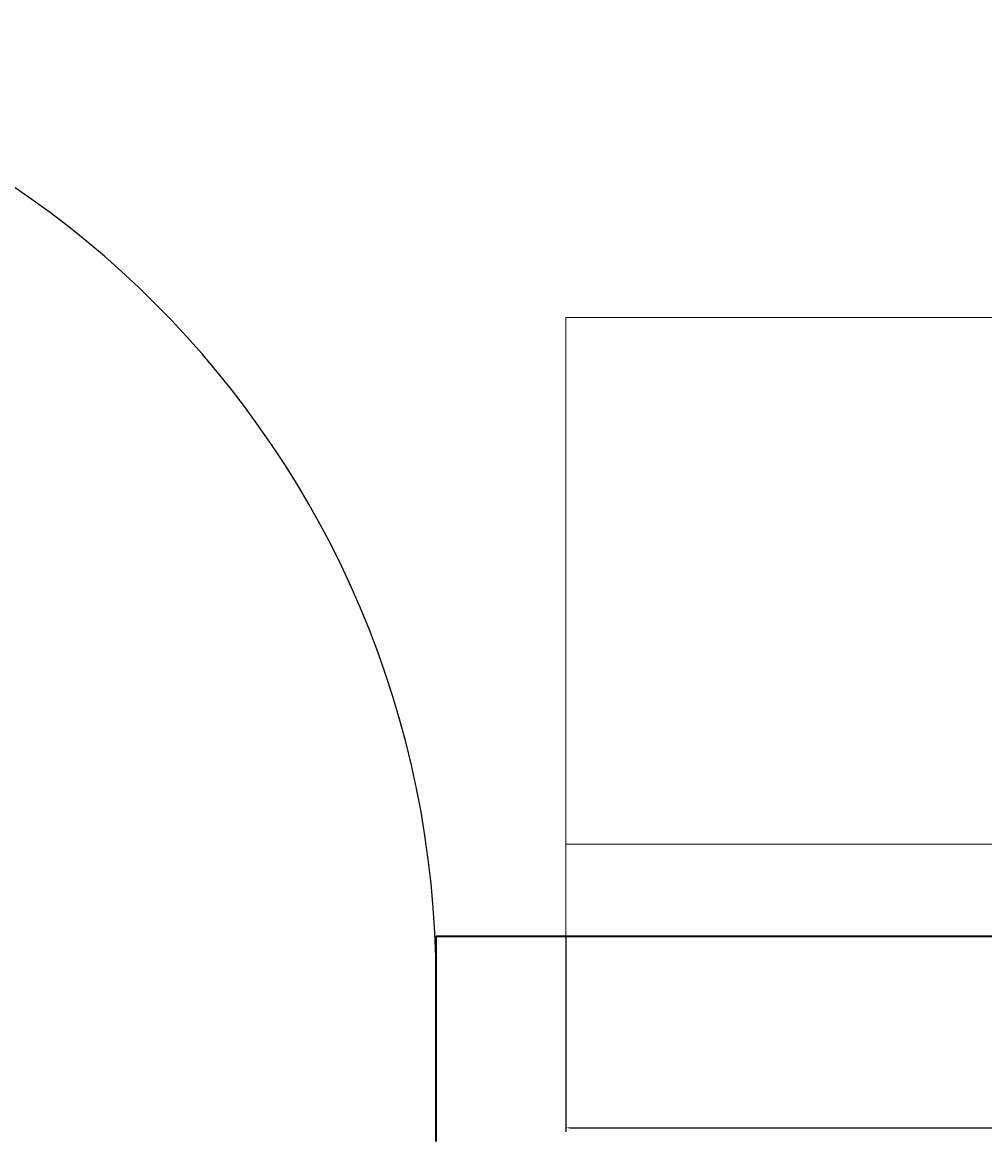
# Model space of a CAD drawing. Units: inches. Extents: x 108 to 613, y 1573 to 2319.
# Tile 4 of 11: x 323 to 365, y 1989 to 2038. Entities that reach past the tile are written whole.
import ezdxf

# ---------------------------------------------------------------- set-up
doc = ezdxf.new("R2010")
doc.units = ezdxf.units.IN
for name, color, linetype, lineweight in [('A-ANNO-DIMS', 2, 'Continuous', 18), ('door', 4, 'Continuous', 25), ('furniture', 2, 'Continuous', 18), ('wall', 6, 'Continuous', 35)]:
    doc.layers.add(name, color=color, linetype=linetype, lineweight=lineweight)
doc.styles.get("Standard").update_dxf_attribs({"font": 'arial.ttf'})
doc.dimstyles.get("Standard").update_dxf_attribs({"dimtxt": 0.18, "dimasz": 0.18, "dimexe": 0.18, "dimexo": 0.0625, "dimgap": 0.09, "dimtad": 0, "dimtih": 1, "dimtoh": 1, "dimdec": 4, "dimzin": 0, "dimdsep": 46, "dimtxsty": 'Standard', "dimcen": 0.09, "dimadec": 0, "dimazin": 0, "dimtfac": 1, "dimtdec": 4, "dimtofl": 0, "dimtmove": 0, "dimatfit": 3, "dimfxl": 1, "dimtolj": 1, "dimtzin": 0, "dimarcsym": 0})

# ---------------------------------------------------------------- blocks, each defined once
blk = doc.blocks.new('*U2')
for p, q in [((0, 0), (0, -5)), ((30, 0), (30, -5))]:
    blk.add_line(p, q)
blk.add_lwpolyline([(0, 0), (0, 30), (1.75, 30), (1.75, 0)], close=True)
blk.add_arc((0, 0), 30, 0, 90)
blk = doc.blocks.new('SOFA-2-SEAT')
for p, q in [((25.991, 27.084), (25.991, 4.025)), ((27.991, 27.084), (27.991, 4.025)), ((55.982, 4.025), (0, 4.025))]:
    blk.add_line(p, q)
blk.add_lwpolyline([(0, 27.084), (55.982, 27.084), (55.982, 0), (0, 0)], close=True)
blk = doc.blocks.new('*D33')
at = {"layer": 'A-ANNO-DIMS', "color": 0, "lineweight": -2, "transparency": 16777216}
for p, q in [((346.962, 1997.55), (346.962, 1989.035)), ((402.944, 1997.55), (402.944, 1989.035)), ((347.142, 1989.215), (373.571, 1989.215)), ((402.764, 1989.215), (376.335, 1989.215))]:
    blk.add_line(p, q, dxfattribs=at)
at = {"layer": 'A-ANNO-DIMS', "color": 0, "transparency": 16777216}
for points in [[(347.142, 1989.245), (347.142, 1989.185), (346.962, 1989.215)], [(402.764, 1989.245), (402.764, 1989.185), (402.944, 1989.215)]]:
    blk.add_solid(points, dxfattribs=at)
at = {"layer": 'Defpoints', "color": 0, "transparency": 16777216}
for p in [(346.962, 1997.612), (402.944, 1997.612), (402.944, 1989.215)]:
    blk.add_point(p, dxfattribs=at)
at = {"layer": 'A-ANNO-DIMS', "color": 0, "transparency": 16777216, "insert": (374.953, 1989.215), "char_height": 0.18, "attachment_point": 5}
blk.add_mtext('\\A1;2-SEAT SOFA 56 TYP.', dxfattribs=at)

msp = doc.modelspace()

# ---------------------------------------------------------------- linework, layer by layer
at = {"layer": 'wall'}
for p, q in [((341.2753, 1997.6125), (431.2753, 1997.6125)), ((341.2753, 1988.6125), (341.2753, 1997.6125))]:
    msp.add_line(p, q, dxfattribs=at)

# ---------------------------------------------------------------- block references
at = {"layer": 'door', "xscale": 1.399999999999996, "yscale": 1.399999999999996, "zscale": 1.399999999999996}
msp.add_blockref('*U2', (299.2753, 1995.6125), dxfattribs=at)
at = {"layer": 'furniture'}
msp.add_blockref('SOFA-2-SEAT', (346.962, 1997.612), dxfattribs=at)

# ---------------------------------------------------------------- dimensions: what is measured, and where the dimension line sits
at = {"layer": 'A-ANNO-DIMS'}
dim = msp.add_linear_dim(base=(402.9438, 1989.2152), p1=(346.9619, 1997.6125), p2=(402.9438, 1997.6125), text='2-SEAT SOFA <> TYP.', dimstyle='Standard', override={"dimdec": 0, "dimlfac": 1, "dimrnd": 0, "dimzin": 0, "dimdsep": 46, "dimlunit": 2}, dxfattribs=at)
dim.commit()
dim.dimension.update_dxf_attribs({"geometry": '*D33', "text_midpoint": (374.9528, 1989.2152)})

doc.saveas('drawing.dxf')
